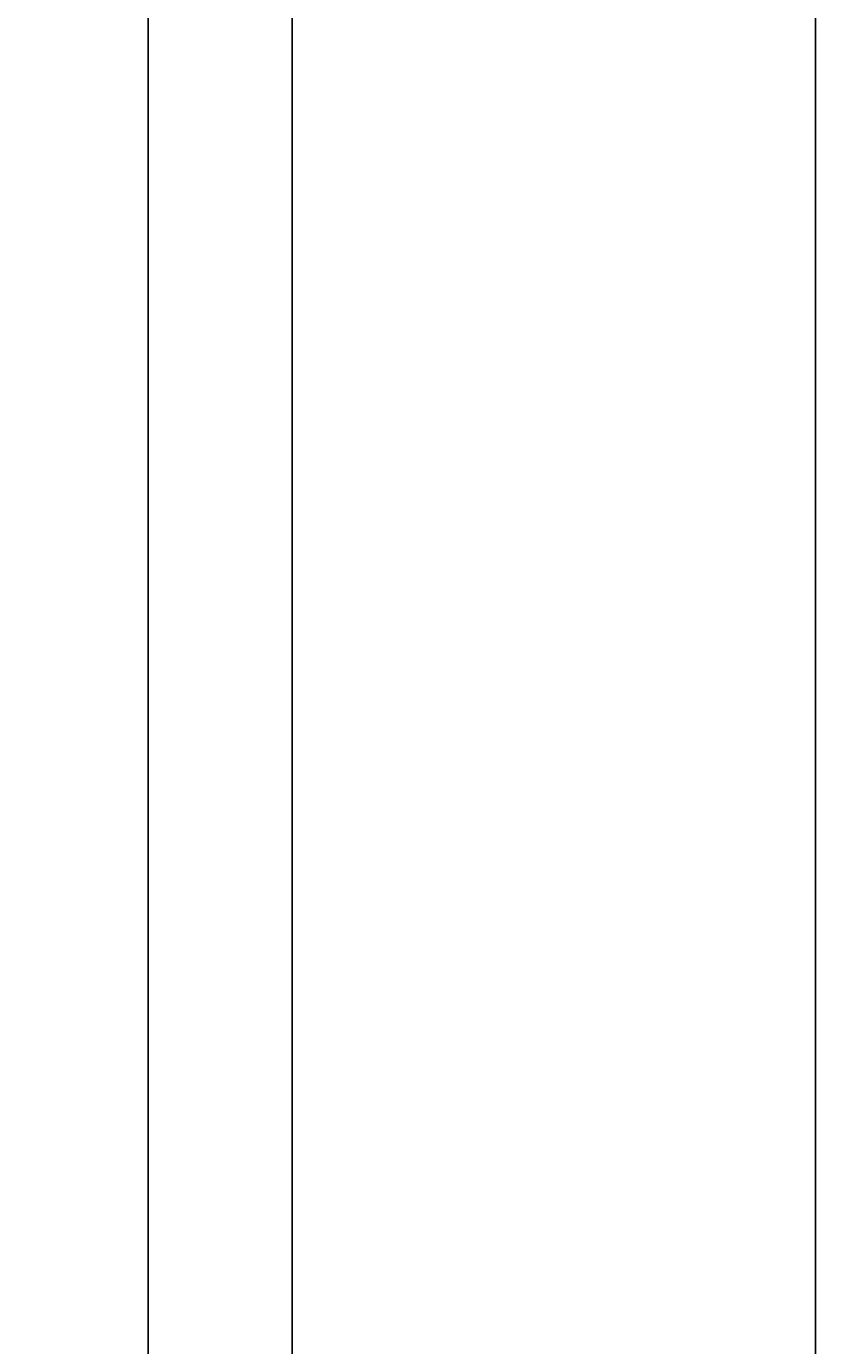
# Model space of a CAD drawing. Units: inches. Extents: x 2812 to 3051, y 1398 to 1659.
# Tile 40 of 65: x 2966 to 2984, y 1498 to 1528. Entities that reach past the tile are written whole.
import ezdxf

# ---------------------------------------------------------------- set-up
doc = ezdxf.new("R2010")
doc.units = ezdxf.units.IN
doc.layers.add('A-ANNO-DIMS', color=2, linetype='Continuous', lineweight=18)
doc.styles.get("Standard").update_dxf_attribs({"font": 'arial.ttf'})
doc.dimstyles.get("Standard").update_dxf_attribs({"dimtxt": 0.18, "dimasz": 0.18, "dimexe": 0.18, "dimexo": 0.0625, "dimgap": 0.09, "dimtad": 0, "dimtih": 1, "dimtoh": 1, "dimdec": 4, "dimzin": 0, "dimdsep": 46, "dimtxsty": 'Standard', "dimcen": 0.09, "dimadec": 0, "dimazin": 0, "dimtfac": 1, "dimtdec": 4, "dimtofl": 0, "dimtmove": 0, "dimatfit": 3, "dimfxl": 1, "dimtolj": 1, "dimtzin": 0, "dimarcsym": 0})

# ---------------------------------------------------------------- blocks, each defined once
blk = doc.blocks.new('*D31')
at = {"layer": 'A-ANNO-DIMS', "color": 0, "lineweight": -2, "transparency": 16777216}
for p, q in [((2972.272, 1594.192), (2972.272, 1397.505)), ((2961.385, 1559.757), (2961.385, 1397.505)), ((2961.565, 1397.685), (2966.373, 1397.685)), ((2972.092, 1397.685), (2967.283, 1397.685))]:
    blk.add_line(p, q, dxfattribs=at)
at = {"layer": 'A-ANNO-DIMS', "color": 0, "transparency": 16777216}
for points in [[(2961.565, 1397.715), (2961.565, 1397.655), (2961.385, 1397.685)], [(2972.092, 1397.715), (2972.092, 1397.655), (2972.272, 1397.685)]]:
    blk.add_solid(points, dxfattribs=at)
at = {"layer": 'Defpoints', "color": 0, "transparency": 16777216}
for p in [(2972.272, 1594.254), (2961.385, 1559.82), (2972.272, 1397.685)]:
    blk.add_point(p, dxfattribs=at)
at = {"layer": 'A-ANNO-DIMS', "color": 0, "transparency": 16777216, "insert": (2966.828, 1397.685), "char_height": 0.18, "attachment_point": 5}
blk.add_mtext('\\A1;10.887', dxfattribs=at)
blk = doc.blocks.new('*D32')
at = {"layer": 'A-ANNO-DIMS', "color": 0, "lineweight": -2, "transparency": 16777216}
for p, q in [((2984.316, 1598.757), (2984.316, 1397.505)), ((2972.272, 1594.192), (2972.272, 1397.505)), ((2972.452, 1397.685), (2977.839, 1397.685)), ((2984.136, 1397.685), (2978.748, 1397.685))]:
    blk.add_line(p, q, dxfattribs=at)
at = {"layer": 'A-ANNO-DIMS', "color": 0, "transparency": 16777216}
for points in [[(2972.452, 1397.715), (2972.452, 1397.655), (2972.272, 1397.685)], [(2984.136, 1397.715), (2984.136, 1397.655), (2984.316, 1397.685)]]:
    blk.add_solid(points, dxfattribs=at)
at = {"layer": 'Defpoints', "color": 0, "transparency": 16777216}
for p in [(2984.316, 1598.82), (2972.272, 1594.254), (2984.316, 1397.685)]:
    blk.add_point(p, dxfattribs=at)
at = {"layer": 'A-ANNO-DIMS', "color": 0, "transparency": 16777216, "insert": (2978.294, 1397.685), "char_height": 0.18, "attachment_point": 5}
blk.add_mtext('\\A1;12.044', dxfattribs=at)
blk = doc.blocks.new('*D69')
at = {"layer": 'A-ANNO-DIMS', "color": 0, "lineweight": -2, "transparency": 16777216}
for p, q in [((2961.385, 1472.098), (2961.385, 1659.35)), ((2968.956, 1467.81), (2968.956, 1659.35)), ((2961.565, 1659.17), (2964.795, 1659.17)), ((2968.776, 1659.17), (2965.546, 1659.17))]:
    blk.add_line(p, q, dxfattribs=at)
at = {"layer": 'A-ANNO-DIMS', "color": 0, "transparency": 16777216}
for points in [[(2961.565, 1659.2), (2961.565, 1659.14), (2961.385, 1659.17)], [(2968.776, 1659.2), (2968.776, 1659.14), (2968.956, 1659.17)]]:
    blk.add_solid(points, dxfattribs=at)
at = {"layer": 'Defpoints', "color": 0, "transparency": 16777216}
for p in [(2968.956, 1659.17), (2961.385, 1472.035), (2968.956, 1467.747)]:
    blk.add_point(p, dxfattribs=at)
at = {"layer": 'A-ANNO-DIMS', "color": 0, "transparency": 16777216, "insert": (2965.17, 1659.17), "char_height": 0.18, "attachment_point": 5}
blk.add_mtext('\\A1;7.571', dxfattribs=at)

msp = doc.modelspace()

# ---------------------------------------------------------------- dimensions: what is measured, and where the dimension line sits
at = {"layer": 'A-ANNO-DIMS'}
for base, p1, p2, picture, middle in [((2968.9558, 1659.17), (2961.3849, 1472.0354), (2968.9558, 1467.7474), '*D69', (2965.1704, 1659.17)), ((2984.3156, 1397.6854), (2972.2716, 1594.2541), (2984.3156, 1598.82), '*D32', (2978.2936, 1397.6854)), ((2972.2716, 1397.6854), (2961.3849, 1559.82), (2972.2716, 1594.2541), '*D31', (2966.8282, 1397.6854))]:
    dim = msp.add_linear_dim(base=base, p1=p1, p2=p2, dimstyle='Standard', override={"dimdec": 3, "dimlfac": 1, "dimrnd": 0, "dimzin": 0, "dimdsep": 46, "dimlunit": 2}, dxfattribs=at)
    dim.commit()
    dim.dimension.update_dxf_attribs({"geometry": picture, "text_midpoint": middle})

doc.saveas('drawing.dxf')
